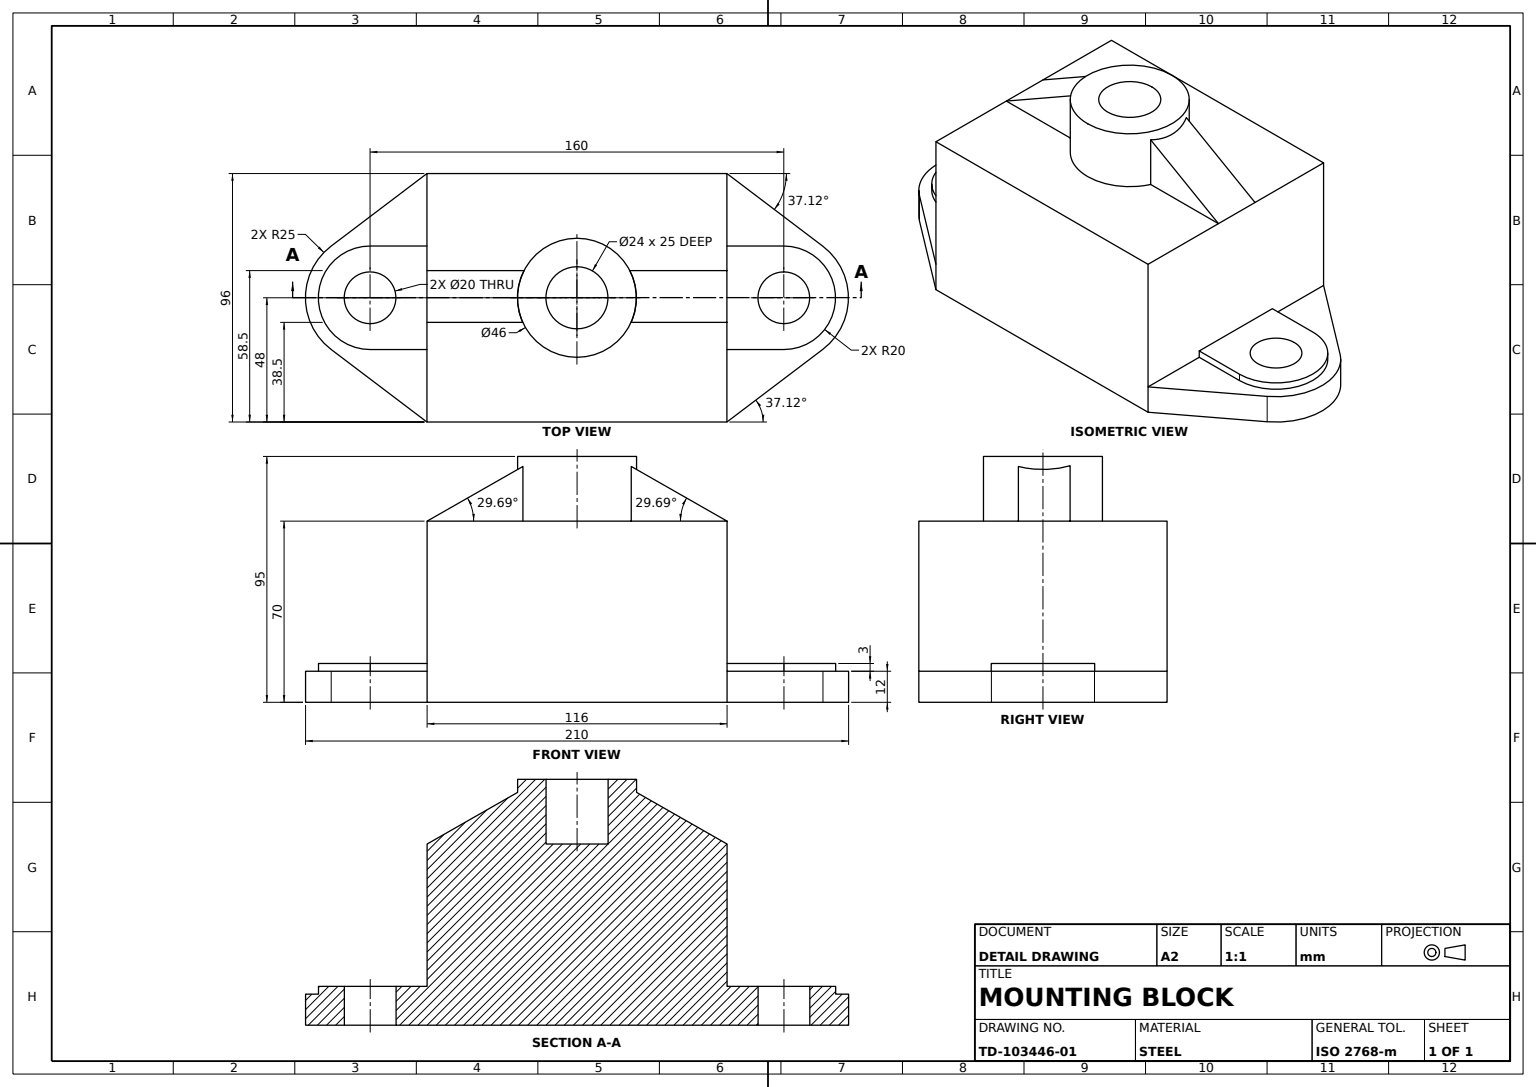
SolidWorks part; units mm, degrees
material "Plain Carbon Steel"
ref_plane "Front Plane" through (0, 0, 0) normal (0, 0, 1) x (1, 0, 0)
ref_plane "Top Plane" through (0, 0, 0) normal (0, 1, 0) x (1, 0, 0)
ref_plane "Right Plane" through (0, 0, 0) normal (1, 0, 0) x (0, 0, -1)
sketch "Housing Block Sketch" plane through (0, 0, 0) normal (0, 0, 1) x (1, 0, 0)
  line L0 (0, 0) -> (116, 0)
  line L1 (116, 0) -> (116, 70)
  line L2 (116, 70) -> (0, 70)
  line L3 (0, 70) -> (0, 0)
  dimension "D1" = 116
  dimension "D2" = 70
extrude "Housing Block" add sketch "Housing Block Sketch" along normal blind 96
ref_plane "Plane1" through (0, 0, 0) normal (0, 1, 0) x (1, 0, 0)
sketch "Mounting Flange Sketch" plane through (0, 0, 0) normal (0, 1, 0) x (1, 0, 0)
  line L0 (116, 0) -> (0, 0) construction
  line L1 (116, 0) -> (116, -96)
  line L2 (116, 0) -> (153.086, -28.0648)
  line L3 (116, -96) -> (153.086, -67.9352)
  arc A0 (153.086, -67.9352) -> (153.086, -28.0648) centre (138, -48) ccw
  point P5 (58, 0)
  dimension "D1" = 50
  dimension "D2" = 48
  dimension "D3" = 80
extrude "Mounting Flange" add sketch "Mounting Flange Sketch" along normal blind 12
sketch "Flange Pad Sketch" plane through (0, 12, 0) normal (0, 1, 0) x (1, 0, 0)
  line L0 (138, -28) -> (116, -28)
  line L1 (116, 0) -> (116, -96) construction
  line L2 (116, -28) -> (116, -68)
  line L3 (116, -96) -> (116, 0) construction
  line L4 (116, -68) -> (138, -68)
  arc A0 (138, -68) -> (138, -28) centre (138, -48) ccw
  dimension "D1" = 40
extrude "Flange Pad" add sketch "Flange Pad Sketch" along normal blind 3
sketch "Flange Hole Sketch" plane through (0, 15, 0) normal (0, 1, 0) x (1, 0, 0)
  circle A0 centre (138, -48) radius 10
  dimension "D1" = 20
extrude "Flange Hole" cut sketch "Flange Hole Sketch" against normal through all
ref_plane "Plane3" through (58, 0, 0) normal (1, 0, 0) x (0, 0, -1)
mirror "Flange Mirror" about plane through (58, 0, 0) normal (1, 0, 0) of "Flange Hole", "Flange Pad", "Mounting Flange"
sketch "Top Boss Sketch" plane through (0, 70, 0) normal (0, 1, 0) x (1, 0, 0)
  line L0 (0, -96) -> (0, 0) construction
  line L1 (116, 0) -> (0, 0) construction
  circle A0 centre (58, -48) radius 23
  circle A1 centre (58, -48) radius 12
  dimension "D1" = 46
  dimension "D2" = 24
  dimension "D3" = 58
  dimension "D4" = 48
extrude "Top Boss Ø46" add sketch "Top Boss Sketch" along normal blind 25
ref_plane "Plane4" through (0, 0, 47.5) normal (0, 0, 1) x (1, 0, 0)
sketch "Gusset Sketch" plane through (0, 0, 47.5) normal (0, 0, 1) x (1, 0, 0)
  line L2 (116, 70) -> (0, 70) construction
  line L3 (81, 70) -> (81, 95) construction
  line L4 (81, 70) -> (116, 70)
  line L5 (81, 70) -> (72.156, 70)
  line L6 (72.156, 70) -> (72.156, 95)
  line L7 (81, 95) -> (35, 95) construction
  line L8 (116, 70) -> (72.156, 95)
  dimension "D1" = 8.844
extrude "Gusset" add sketch "Gusset Sketch" along normal mid plane 20
ref_plane "Plane5" through (58, 0, 0) normal (1, 0, 0) x (0, 0, -1)
mirror "Gusset Mirror" about plane through (58, 0, 0) normal (1, 0, 0) of "Gusset"
